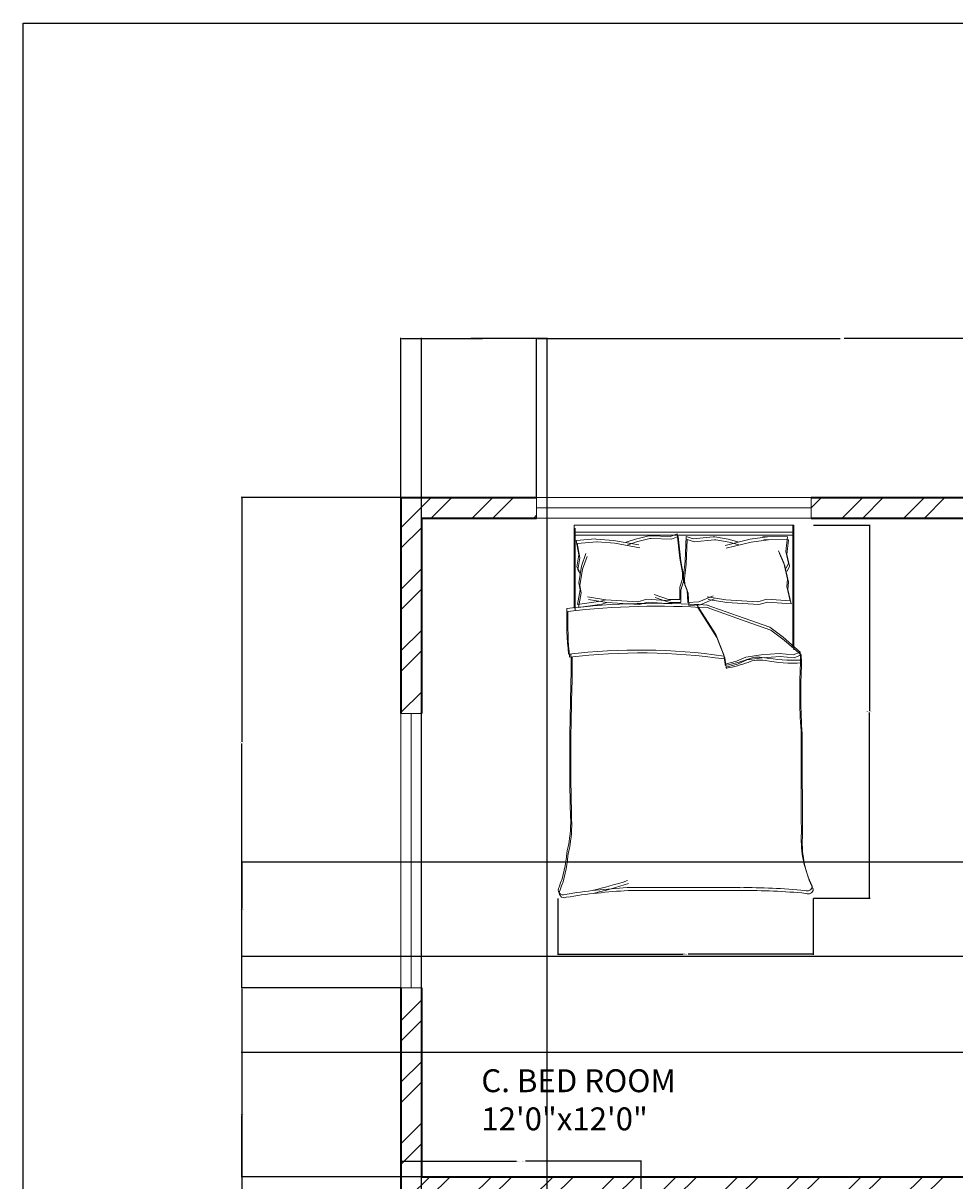
# Model space of a CAD drawing. Units: inches. Extents: x 1965 to 2673, y 1802 to 2669.
# Tile 9 of 16: x 1965 to 2168, y 2416 to 2669. Entities that reach past the tile are written whole.
import ezdxf

# ---------------------------------------------------------------- set-up
doc = ezdxf.new("R2010")
doc.units = ezdxf.units.IN
for name, color, linetype, lineweight in [('A-ANNO-DIMS', 2, 'Continuous', 18), ('A-ANNO-TTLB', 7, 'Continuous', 25), ('A-AREA-IDEN', 7, 'Continuous', 18), ('A-FURN', 8, 'Continuous', 13), ('A-GLAZ', 181, 'Continuous', 18), ('A-WALL', 7, 'Continuous', 35), ('A-WALL-PATT', 252, 'Continuous', 13)]:
    doc.layers.add(name, color=color, linetype=linetype, lineweight=lineweight)
doc.styles.get("Standard").update_dxf_attribs({"font": 'arial.ttf'})
doc.dimstyles.get("Standard").update_dxf_attribs({"dimtxt": 0.18, "dimasz": 0.18, "dimexe": 0.18, "dimexo": 0.0625, "dimgap": 0.09, "dimtad": 0, "dimtih": 1, "dimtoh": 1, "dimdec": 4, "dimzin": 0, "dimdsep": 46, "dimtxsty": 'Standard', "dimcen": 0.09, "dimadec": 0, "dimazin": 0, "dimtfac": 1, "dimtdec": 4, "dimtofl": 0, "dimtmove": 0, "dimatfit": 3, "dimfxl": 1, "dimtolj": 1, "dimtzin": 0, "dimarcsym": 0})

# ---------------------------------------------------------------- blocks, each defined once
blk = doc.blocks.new('BED-DOUBLE')
for p, q in [((3.47, 63.33), (3.47, 81.44)), ((3.47, 63.33), (3.47, 81.44)), ((3.47, 81.44), (51.49, 81.44)), ((51.26, 81.44), (51.26, 54.83)), ((51.26, 81.44), (51.26, 54.83)), ((51.49, 81.44), (51.49, 80.8)), ((3.47, 79.91), (51.26, 79.91)), ((3.47, 79.91), (51.26, 79.91)), ((3.7, 62.69), (3.7, 80.8)), ((3.7, 62.69), (3.7, 80.8)), ((3.7, 79.27), (51.49, 79.27)), ((3.7, 79.27), (51.49, 79.27)), ((16.87, 78.41), (19.76, 79.14)), ((16.87, 78.41), (19.76, 79.14)), ((17.1, 77.77), (19.99, 78.5)), ((17.1, 77.77), (19.99, 78.5)), ((19.76, 79.14), (20.09, 79.14)), ((19.76, 79.14), (20.09, 79.14)), ((19.99, 78.5), (20.31, 78.5)), ((19.99, 78.5), (20.31, 78.5)), ((20.09, 79.14), (24.53, 78.99)), ((20.09, 79.14), (24.53, 78.99)), ((20.31, 78.5), (24.76, 78.35)), ((20.31, 78.5), (24.76, 78.35)), ((24.53, 78.99), (25.98, 79.57)), ((24.53, 78.99), (25.98, 79.57)), ((24.76, 78.35), (26.21, 78.93)), ((24.76, 78.35), (26.21, 78.93)), ((25.98, 79.57), (26.56, 74.22)), ((25.98, 79.57), (26.56, 74.22)), ((26.21, 78.93), (26.78, 73.58)), ((26.21, 78.93), (26.78, 73.58)), ((27.97, 78.95), (27.73, 73.57)), ((27.97, 78.95), (27.73, 73.57)), ((29.45, 78.46), (27.97, 78.95)), ((29.45, 78.46), (27.97, 78.95)), ((33.88, 78.88), (29.45, 78.46)), ((33.88, 78.88), (29.45, 78.46)), ((34.2, 78.9), (33.88, 78.88)), ((34.2, 78.9), (33.88, 78.88)), ((37.13, 78.36), (34.2, 78.9)), ((37.13, 78.36), (34.2, 78.9)), ((45.71, 78.9), (41.91, 78.37)), ((45.71, 78.9), (41.91, 78.37)), ((50.11, 78.88), (44.7, 78.98)), ((44.7, 78.98), (45.71, 78.9)), ((50.11, 78.88), (44.7, 78.98)), ((44.7, 78.98), (45.71, 78.9)), ((50.11, 78.88), (49.73, 75.67)), ((50.11, 78.88), (49.73, 75.67)), ((51.49, 80.8), (51.49, 54.19)), ((51.49, 80.8), (51.49, 54.19)), ((3.89, 78.1), (8.17, 78.43)), ((3.89, 78.1), (8.17, 78.43)), ((3.89, 78.12), (4.47, 74.94)), ((3.89, 78.12), (4.47, 74.94)), ((4.12, 77.46), (8.4, 77.79)), ((4.12, 77.46), (8.4, 77.79)), ((4.12, 77.49), (4.7, 74.3)), ((4.12, 77.49), (4.7, 74.3)), ((8.17, 78.43), (8.28, 78.41)), ((8.17, 78.43), (8.28, 78.41)), ((8.28, 78.41), (12.1, 78.12)), ((8.28, 78.41), (12.1, 78.12)), ((8.4, 77.79), (8.51, 77.77)), ((8.4, 77.79), (8.51, 77.77)), ((8.51, 77.77), (12.33, 77.49)), ((8.51, 77.77), (12.33, 77.49)), ((12.1, 78.12), (17.6, 77.11)), ((12.1, 78.12), (17.6, 77.11)), ((12.33, 77.49), (17.82, 76.47)), ((12.33, 77.49), (17.82, 76.47)), ((14.85, 77.69), (16.87, 78.41)), ((14.85, 77.69), (16.87, 78.41)), ((15.08, 77.05), (17.1, 77.77)), ((15.08, 77.05), (17.1, 77.77)), ((28.2, 78.31), (27.96, 72.93)), ((28.2, 78.31), (27.96, 72.93)), ((29.68, 77.82), (28.2, 78.31)), ((29.68, 77.82), (28.2, 78.31)), ((34.11, 78.24), (29.68, 77.82)), ((34.11, 78.24), (29.68, 77.82)), ((34.43, 78.26), (34.11, 78.24)), ((34.43, 78.26), (34.11, 78.24)), ((37.36, 77.72), (34.43, 78.26)), ((37.36, 77.72), (34.43, 78.26)), ((41.91, 78.37), (36.49, 77.02)), ((41.91, 78.37), (36.49, 77.02)), ((42.14, 77.73), (36.72, 76.38)), ((42.14, 77.73), (36.72, 76.38)), ((39.2, 77.77), (37.13, 78.36)), ((39.19, 77.77), (37.13, 78.36)), ((39.42, 77.13), (37.36, 77.72)), ((39.42, 77.13), (37.36, 77.72)), ((45.94, 78.26), (42.14, 77.73)), ((45.94, 78.26), (42.14, 77.73)), ((50.34, 78.24), (44.93, 78.34)), ((44.93, 78.34), (45.94, 78.26)), ((50.34, 78.24), (44.93, 78.34)), ((44.93, 78.34), (45.94, 78.26)), ((50.34, 78.24), (49.96, 75.03)), ((50.34, 78.24), (49.96, 75.03)), ((4.47, 74.94), (4.03, 72.34)), ((4.47, 74.94), (4.03, 72.34)), ((4.7, 74.3), (4.26, 71.7)), ((4.7, 74.3), (4.26, 71.7)), ((5.05, 72.49), (6.06, 75.23)), ((5.05, 72.49), (6.06, 75.23)), ((5.27, 71.85), (6.29, 74.59)), ((5.27, 71.85), (6.29, 74.59)), ((26.56, 74.22), (27.13, 71.04)), ((26.56, 74.22), (27.13, 71.04)), ((26.78, 73.58), (27.36, 70.4)), ((26.78, 73.58), (27.36, 70.4)), ((27.73, 73.57), (27.35, 70.36)), ((27.73, 73.57), (27.35, 70.36)), ((49.3, 73.18), (48.12, 75.86)), ((49.3, 73.18), (48.12, 75.86)), ((49.53, 72.54), (48.35, 75.22)), ((49.53, 72.54), (48.35, 75.22)), ((49.73, 75.67), (50.32, 73.1)), ((49.73, 75.67), (50.32, 73.1)), ((49.96, 75.03), (50.55, 72.46)), ((49.96, 75.03), (50.55, 72.46)), ((4.03, 72.34), (4.61, 71.33)), ((4.03, 72.34), (4.61, 71.33)), ((4.26, 71.7), (4.84, 70.69)), ((4.26, 71.7), (4.84, 70.69)), ((4.47, 68.87), (5.05, 72.49)), ((4.47, 68.87), (5.05, 72.49)), ((4.7, 68.23), (5.27, 71.85)), ((4.7, 68.23), (5.27, 71.85)), ((27.13, 71.04), (27.13, 69.74)), ((27.13, 71.04), (27.13, 69.74)), ((27.96, 72.93), (27.58, 69.72)), ((27.96, 72.93), (27.58, 69.72)), ((50.11, 69.61), (49.3, 73.18)), ((50.11, 69.61), (49.3, 73.18)), ((50.34, 68.97), (49.53, 72.54)), ((50.34, 68.97), (49.53, 72.54)), ((50.32, 73.1), (49.81, 72.06)), ((50.32, 73.1), (49.81, 72.06)), ((50.55, 72.46), (50.04, 71.42)), ((50.55, 72.46), (50.04, 71.42)), ((4.76, 67.28), (4.47, 68.87)), ((4.76, 67.28), (4.47, 68.87)), ((27.13, 69.74), (26.56, 67.86)), ((27.13, 69.74), (26.56, 67.86)), ((27.36, 69.1), (26.78, 67.22)), ((27.36, 69.1), (26.78, 67.22)), ((27.35, 70.36), (27.43, 69.06)), ((27.35, 70.36), (27.43, 69.06)), ((27.36, 70.4), (27.36, 69.1)), ((27.36, 70.4), (27.36, 69.1)), ((27.43, 69.06), (28.13, 67.22)), ((27.43, 69.06), (28.13, 67.22)), ((27.58, 69.72), (27.66, 68.42)), ((27.58, 69.72), (27.66, 68.42)), ((27.66, 68.42), (28.35, 66.58)), ((27.66, 68.42), (28.35, 66.58)), ((49.92, 68.01), (50.11, 69.61)), ((49.92, 68.01), (50.11, 69.61)), ((50.15, 67.37), (50.34, 68.97)), ((50.15, 67.37), (50.34, 68.97)), ((4.18, 64.1), (4.76, 67.28)), ((4.18, 64.1), (4.76, 67.28)), ((4.41, 63.46), (4.99, 66.64)), ((4.41, 63.46), (4.99, 66.64)), ((4.99, 66.64), (4.7, 68.23)), ((4.99, 66.64), (4.7, 68.23)), ((6.38, 65.81), (10.41, 65.15)), ((6.38, 65.81), (10.41, 65.15)), ((24.1, 65.18), (20.95, 66.27)), ((24.1, 65.18), (20.95, 66.27)), ((26.56, 67.86), (26.56, 65.18)), ((26.56, 67.86), (26.56, 65.18)), ((26.78, 67.22), (26.78, 64.54)), ((26.78, 67.22), (26.78, 64.54)), ((28.13, 67.22), (28.29, 64.55)), ((28.13, 67.22), (28.29, 64.55)), ((28.35, 66.58), (28.52, 63.91)), ((28.35, 66.58), (28.52, 63.91)), ((30.75, 64.7), (33.82, 65.99)), ((30.75, 64.7), (33.82, 65.99)), ((32.56, 65.81), (36.59, 65.15)), ((32.56, 65.81), (36.59, 65.15)), ((50.69, 64.87), (49.92, 68.01)), ((50.69, 64.87), (49.92, 68.01)), ((50.92, 64.23), (50.15, 67.37)), ((50.92, 64.23), (50.15, 67.37)), ((9.28, 64.82), (4.18, 64.1)), ((9.28, 64.82), (4.18, 64.1)), ((9.5, 64.18), (4.41, 63.46)), ((9.5, 64.18), (4.41, 63.46)), ((6.6, 65.17), (10.64, 64.51)), ((6.61, 65.17), (10.64, 64.51)), ((10.41, 65.15), (9.28, 64.82)), ((10.41, 65.15), (9.28, 64.82)), ((10.64, 64.51), (9.5, 64.18)), ((10.64, 64.51), (9.5, 64.18)), ((10.41, 65.15), (17.42, 64.71)), ((10.41, 65.15), (17.42, 64.71)), ((10.64, 64.51), (17.65, 64.08)), ((10.64, 64.51), (17.65, 64.08)), ((17.42, 64.71), (19.38, 65.27)), ((17.42, 64.71), (19.38, 65.27)), ((17.65, 64.08), (19.61, 64.63)), ((17.65, 64.08), (19.61, 64.63)), ((19.38, 65.27), (24.51, 64.87)), ((19.38, 65.27), (24.51, 64.87)), ((19.61, 64.63), (24.74, 64.23)), ((19.61, 64.63), (24.74, 64.23)), ((24.33, 64.54), (21.18, 65.63)), ((24.33, 64.54), (21.18, 65.63)), ((26.56, 65.18), (24.1, 65.18)), ((26.56, 65.18), (24.1, 65.18)), ((26.78, 64.54), (24.33, 64.54)), ((26.78, 64.54), (24.33, 64.54)), ((28.29, 64.55), (30.75, 64.7)), ((28.29, 64.55), (30.75, 64.7)), ((28.52, 63.91), (30.97, 64.06)), ((28.52, 63.91), (30.97, 64.06)), ((30.25, 64.06), (34.44, 57.56)), ((30.25, 64.06), (34.44, 57.56)), ((30.48, 63.42), (34.67, 56.92)), ((30.48, 63.42), (34.67, 56.92)), ((30.97, 64.06), (34.04, 65.35)), ((30.97, 64.06), (34.04, 65.35)), ((40.64, 61.12), (32.3, 64.06)), ((40.64, 61.12), (32.3, 64.06)), ((40.87, 60.48), (32.53, 63.42)), ((40.87, 60.48), (32.53, 63.42)), ((32.79, 65.17), (36.82, 64.51)), ((32.79, 65.17), (36.82, 64.51)), ((36.59, 65.15), (43.6, 64.71)), ((36.59, 65.15), (43.6, 64.71)), ((36.82, 64.51), (43.83, 64.08)), ((36.82, 64.51), (43.83, 64.08)), ((43.6, 64.71), (45.56, 65.27)), ((43.6, 64.71), (45.56, 65.27)), ((43.83, 64.08), (45.79, 64.63)), ((43.83, 64.08), (45.79, 64.63)), ((45.56, 65.27), (50.69, 64.87)), ((45.56, 65.27), (50.69, 64.87)), ((45.79, 64.63), (50.92, 64.23)), ((45.79, 64.63), (50.92, 64.23)), ((46.21, 59.11), (40.64, 61.12)), ((46.21, 59.11), (40.64, 61.12)), ((46.44, 58.47), (40.87, 60.48)), ((46.44, 58.47), (40.87, 60.48)), ((49.16, 56.95), (46.21, 59.11)), ((49.16, 56.95), (46.21, 59.11)), ((49.39, 56.31), (46.44, 58.47)), ((49.39, 56.31), (46.44, 58.47)), ((34.44, 57.56), (36.15, 53.08)), ((34.44, 57.56), (36.15, 53.08)), ((34.67, 56.92), (36.38, 52.44)), ((34.67, 56.92), (36.38, 52.44)), ((52.86, 53.69), (49.16, 56.95)), ((52.86, 53.69), (49.16, 56.95)), ((53.09, 53.06), (49.39, 56.31)), ((53.09, 53.06), (49.39, 56.31)), ((44.36, 53.08), (48.23, 53.39)), ((44.36, 53.08), (48.23, 53.39)), ((48.23, 53.39), (51.33, 53.08)), ((48.23, 53.39), (51.33, 53.08)), ((51.33, 53.08), (52.86, 53.69)), ((51.33, 53.08), (52.86, 53.69)), ((52.94, 51.95), (52.86, 53.69, 3.87)), ((52.94, 51.95), (52.86, 53.69, 3.87)), ((36.15, 53.08), (36.46, 51.06)), ((36.15, 53.08), (36.46, 51.06)), ((36.38, 52.44), (36.69, 50.42)), ((36.38, 52.44), (36.69, 50.42)), ((36.46, 51.06), (38.94, 51.68)), ((36.46, 51.06), (38.94, 51.68)), ((36.69, 50.42), (39.16, 51.04)), ((36.69, 50.42), (39.16, 51.04)), ((38.94, 51.68), (40.95, 52.61)), ((38.94, 51.68), (40.95, 52.61)), ((39.16, 51.04), (41.18, 51.97)), ((39.16, 51.04), (41.18, 51.97)), ((40.95, 52.61), (44.36, 53.08)), ((40.95, 52.61), (44.36, 53.08)), ((41.18, 51.97), (44.58, 52.44)), ((41.18, 51.97), (44.58, 52.44)), ((44.58, 52.44), (48.46, 52.75)), ((44.58, 52.44), (48.46, 52.75)), ((48.46, 52.75), (51.55, 52.44)), ((48.46, 52.75), (51.55, 52.44)), ((51.55, 52.44), (53.09, 53.06)), ((51.55, 52.44), (53.09, 53.06)), ((53.17, 51.31), (53.09, 53.06, 3.87)), ((53.17, 51.31), (53.09, 53.06, 3.87)), ((15.06, 2.2), (39.67, 2.2)), ((15.06, 2.2), (39.67, 2.2)), ((15.29, 1.56), (39.9, 1.56)), ((15.29, 1.56), (39.9, 1.56))]:
    blk.add_line(p, q)
for centre, radius, start, end in [((21.35, -100.61), 164.97, 86.0865, 96.7821), ((21.35, -100.61), 164.97, 86.0865, 96.7821), ((21.58, -101.25), 164.97, 86.0865, 96.7821), ((21.58, -101.25), 164.97, 86.0865, 96.7821), ((85.16, 61.34), 83.31, 178.7218, 185.604), ((85.16, 61.34), 83.31, 178.7218, 185.604), ((85.39, 60.71), 83.31, 178.7218, 185.604), ((85.38, 60.71), 83.31, 178.7218, 185.604), ((17.75, -74.88), 129.02, 81.7845, 96.9006), ((17.75, -74.88), 129.02, 81.7845, 96.9006), ((17.98, -75.51), 129.02, 81.7845, 96.9006), ((17.98, -75.51), 129.02, 81.7845, 96.9006), ((-167.31, 50.27), 170.11, 358.4762, 1.0082), ((-167.31, 50.27), 170.11, 358.4762, 1.0082), ((-167.08, 49.63), 170.11, 358.4762, 1.0082), ((-167.08, 49.63), 170.11, 358.4762, 1.0082), ((36.63, 51), 0.185, 160.2464, 271.1377), ((36.63, 51), 0.185, 160.2464, 271.1377), ((31.15, 79.96), 29.65, 280.6617, 289.8806), ((31.15, 79.96), 29.65, 280.6617, 289.8806), ((31.38, 79.32), 29.65, 280.6617, 289.8806), ((31.38, 79.32), 29.65, 280.6617, 289.8806), ((43.74, 46.37), 6.22, 78.6608, 113.7384), ((43.74, 46.37), 6.22, 78.6608, 113.7384), ((43.97, 45.74), 6.22, 78.6608, 113.7384), ((43.97, 45.74), 6.22, 78.6608, 113.7384), ((51.32, 88.1), 36.18, 259.8763, 272.5657), ((51.32, 88.1), 36.18, 259.8763, 272.5657), ((51.55, 87.46), 36.18, 259.8763, 272.5657), ((51.55, 87.46), 36.18, 259.8763, 272.5657), ((182.26, 45.13), 129.5, 176.9791, 183.8365), ((182.26, 45.13), 129.5, 176.9791, 183.8365), ((182.49, 44.49), 129.5, 176.9791, 183.8365), ((182.49, 44.49), 129.5, 176.9791, 183.8365), ((36.86, 50.36), 0.185, 160.2464, 271.1377), ((36.86, 50.36), 0.185, 160.2464, 271.1377), ((484.82, 30.83), 482.31, 178.2277, 181.7185), ((484.82, 30.83), 482.31, 178.2277, 181.7185), ((485.05, 30.19), 482.31, 178.2277, 181.7185), ((485.05, 30.19), 482.31, 178.2277, 181.7185), ((-4508.75, 13.62), 4561.86, 0.00217, 0.28689), ((-4508.75, 13.62), 4561.86, 0.00217, 0.28689), ((-4508.52, 12.98), 4561.86, 0.00217, 0.28689), ((-4508.52, 12.98), 4561.86, 0.00217, 0.28689), ((-26.9, 16.93), 29.63, 346.0648, 358.9113), ((-26.9, 16.93), 29.63, 346.0648, 358.9113), ((-26.68, 16.29), 29.63, 346.0648, 358.9113), ((-26.68, 16.29), 29.63, 346.0648, 358.9113), ((76.15, 12.77), 23.07, 177.4714, 206.4681), ((76.15, 12.77), 23.07, 177.4714, 206.4681), ((76.38, 12.14), 23.07, 177.4714, 206.4681), ((76.38, 12.14), 23.07, 177.4714, 206.4681), ((-21.66, 11.17), 23.56, 337.9751, 356.652), ((-21.66, 11.17), 23.56, 337.9751, 356.652), ((-21.44, 10.53), 23.56, 337.9751, 356.652), ((-21.44, 10.53), 23.56, 337.9751, 356.652), ((-17.23, 105.15), 106.46, 283.3832, 287.7053), ((-17.23, 105.15), 106.46, 283.3832, 287.7053), ((-17, 104.51), 106.46, 283.3832, 287.7053), ((-17, 104.51), 106.46, 283.3832, 287.7053), ((1.08, 1.72), 1.09, 146.1736, 293.4781), ((1.08, 1.72), 1.09, 146.1736, 293.4781), ((1.31, 1.08), 1.09, 146.1736, 293.4781), ((1.31, 1.08), 1.09, 146.1736, 293.4781), ((21.42, -119.4), 121.76, 92.9958, 99.4091), ((21.42, -119.4), 121.76, 92.9958, 99.4091), ((21.65, -120.04), 121.76, 92.9958, 99.4091), ((21.65, -120.04), 121.76, 92.9958, 99.4091), ((41.15, -130.84), 133.04, 84.4998, 90.6351), ((41.15, -130.84), 133.04, 84.4998, 90.6351), ((41.38, -131.48), 133.04, 84.4998, 90.6351), ((41.37, -131.48), 133.04, 84.4998, 90.6351), ((54.4, 2.57), 1.1, 242.6588, 356.02), ((54.4, 2.57), 1.1, 242.6588, 356.02), ((54.63, 1.93), 1.1, 242.6588, 356.02), ((54.63, 1.93), 1.1, 242.6588, 356.02)]:
    blk.add_arc(centre, radius, start, end)
blk = doc.blocks.new('WIN-60IN')
for p, q in [((0, 4.5), (0, 0)), ((0, 4.5), (60, 4.5)), ((60, 2.25), (60, 4.5)), ((60, 4.5), (60, 0)), ((0, 0), (0, 2.25)), ((0, 2.25), (60, 2.25)), ((60, 0), (0, 0))]:
    blk.add_line(p, q)
blk = doc.blocks.new('*D15')
at = {"layer": 'A-ANNO-DIMS', "color": 0, "lineweight": -2, "transparency": 16777216}
for p, q in [((2137.28, 2559.53), (2149.63, 2559.53)), ((2149.45, 2559.35), (2149.45, 2518.94)), ((2149.45, 2478.16), (2149.45, 2518.57)), ((2137.28, 2477.98), (2149.63, 2477.98))]:
    blk.add_line(p, q, dxfattribs=at)
at = {"layer": 'A-ANNO-DIMS', "color": 0, "transparency": 16777216}
for points in [[(2149.42, 2559.35), (2149.48, 2559.35), (2149.45, 2559.53)], [(2149.42, 2478.16), (2149.48, 2478.16), (2149.45, 2477.98)]]:
    blk.add_solid(points, dxfattribs=at)
at = {"layer": 'Defpoints', "color": 0, "transparency": 16777216}
for p in [(2137.21, 2559.53), (2149.45, 2559.53), (2137.21, 2477.98)]:
    blk.add_point(p, dxfattribs=at)
at = {"layer": 'A-ANNO-DIMS', "color": 0, "transparency": 16777216, "insert": (2149.45, 2518.76), "char_height": 0.18, "attachment_point": 5}
blk.add_mtext('\\A1;BED 82 TYP.', dxfattribs=at)
blk = doc.blocks.new('*D16')
at = {"layer": 'A-ANNO-DIMS', "color": 0, "lineweight": -2, "transparency": 16777216}
for p, q in [((2081.39, 2477.92), (2081.39, 2465.57)), ((2137.21, 2477.92), (2137.21, 2465.57)), ((2081.57, 2465.75), (2108.77, 2465.75)), ((2137.03, 2465.75), (2109.83, 2465.75))]:
    blk.add_line(p, q, dxfattribs=at)
at = {"layer": 'A-ANNO-DIMS', "color": 0, "transparency": 16777216}
for points in [[(2081.57, 2465.78), (2081.57, 2465.72), (2081.39, 2465.75)], [(2137.03, 2465.78), (2137.03, 2465.72), (2137.21, 2465.75)]]:
    blk.add_solid(points, dxfattribs=at)
at = {"layer": 'Defpoints', "color": 0, "transparency": 16777216}
for p in [(2081.39, 2477.98), (2137.21, 2477.98), (2137.21, 2465.75)]:
    blk.add_point(p, dxfattribs=at)
at = {"layer": 'A-ANNO-DIMS', "color": 0, "transparency": 16777216, "insert": (2109.3, 2465.75), "char_height": 0.18, "attachment_point": 5}
blk.add_mtext('\\A1;56 TYP.', dxfattribs=at)
blk = doc.blocks.new('*D23')
at = {"layer": 'A-ANNO-DIMS', "color": 0, "lineweight": -2, "transparency": 16777216}
for p, q in [((2047.09, 2412.65), (2047.09, 2420.65)), ((2047.27, 2420.47), (2072.37, 2420.47)), ((2099.41, 2420.47), (2074.32, 2420.47)), ((2099.59, 2412.65), (2099.59, 2420.65))]:
    blk.add_line(p, q, dxfattribs=at)
at = {"layer": 'A-ANNO-DIMS', "color": 0, "transparency": 16777216}
for points in [[(2047.27, 2420.5), (2047.27, 2420.44), (2047.09, 2420.47)], [(2099.41, 2420.5), (2099.41, 2420.44), (2099.59, 2420.47)]]:
    blk.add_solid(points, dxfattribs=at)
at = {"layer": 'Defpoints', "color": 0, "transparency": 16777216}
for p in [(2099.59, 2420.47), (2047.09, 2412.59), (2099.59, 2412.59)]:
    blk.add_point(p, dxfattribs=at)
at = {"layer": 'A-ANNO-DIMS', "color": 0, "transparency": 16777216, "insert": (2073.34, 2420.47), "char_height": 0.18, "attachment_point": 5}
blk.add_mtext('\\A1;SHAFT 53 TYP.', dxfattribs=at)
blk = doc.blocks.new('*D27')
at = {"layer": 'A-ANNO-DIMS', "color": 0, "lineweight": -2, "transparency": 16777216}
for p, q in [((2047.09, 2565.65), (2047.09, 2600.5)), ((2047.27, 2600.32), (2061.46, 2600.32)), ((2076.58, 2600.32), (2062.39, 2600.32)), ((2076.76, 2565.65), (2076.76, 2600.5))]:
    blk.add_line(p, q, dxfattribs=at)
at = {"layer": 'A-ANNO-DIMS', "color": 0, "transparency": 16777216}
for points in [[(2047.27, 2600.35), (2047.27, 2600.29), (2047.09, 2600.32)], [(2076.58, 2600.35), (2076.58, 2600.29), (2076.76, 2600.32)]]:
    blk.add_solid(points, dxfattribs=at)
at = {"layer": 'Defpoints', "color": 0, "transparency": 16777216}
for p in [(2076.76, 2600.32), (2047.09, 2565.59), (2076.76, 2565.59)]:
    blk.add_point(p, dxfattribs=at)
at = {"layer": 'A-ANNO-DIMS', "color": 0, "transparency": 16777216, "insert": (2061.92, 2600.32), "char_height": 0.18, "attachment_point": 5}
blk.add_mtext('\\A1;29.663', dxfattribs=at)
blk = doc.blocks.new('*D28')
at = {"layer": 'A-ANNO-DIMS', "color": 0, "lineweight": -2, "transparency": 16777216}
for p, q in [((2076.76, 2565.65), (2076.76, 2600.5)), ((2076.94, 2600.32), (2143.04, 2600.32)), ((2210.05, 2600.32), (2143.95, 2600.32)), ((2210.23, 2565.65), (2210.23, 2600.5))]:
    blk.add_line(p, q, dxfattribs=at)
at = {"layer": 'A-ANNO-DIMS', "color": 0, "transparency": 16777216}
for points in [[(2076.94, 2600.35), (2076.94, 2600.29), (2076.76, 2600.32)], [(2210.05, 2600.35), (2210.05, 2600.29), (2210.23, 2600.32)]]:
    blk.add_solid(points, dxfattribs=at)
at = {"layer": 'Defpoints', "color": 0, "transparency": 16777216}
for p in [(2210.23, 2600.32), (2076.76, 2565.59), (2210.23, 2565.59)]:
    blk.add_point(p, dxfattribs=at)
at = {"layer": 'A-ANNO-DIMS', "color": 0, "transparency": 16777216, "insert": (2143.49, 2600.32), "char_height": 0.18, "attachment_point": 5}
blk.add_mtext('\\A1;133.48', dxfattribs=at)
blk = doc.blocks.new('*D37')
at = {"layer": 'A-ANNO-DIMS', "color": 0, "lineweight": -2, "transparency": 16777216}
for p, q in [((2047.03, 2458.38), (2012.19, 2458.38)), ((2012.37, 2458.2), (2012.37, 2383.91)), ((2012.37, 2309.25), (2012.37, 2383.54)), ((2047.03, 2309.07), (2012.19, 2309.07))]:
    blk.add_line(p, q, dxfattribs=at)
at = {"layer": 'A-ANNO-DIMS', "color": 0, "transparency": 16777216}
for points in [[(2012.34, 2458.2), (2012.4, 2458.2), (2012.37, 2458.38)], [(2012.34, 2309.25), (2012.4, 2309.25), (2012.37, 2309.07)]]:
    blk.add_solid(points, dxfattribs=at)
at = {"layer": 'Defpoints', "color": 0, "transparency": 16777216}
for p in [(2012.37, 2458.38), (2047.09, 2458.38), (2047.09, 2309.07)]:
    blk.add_point(p, dxfattribs=at)
at = {"layer": 'A-ANNO-DIMS', "color": 0, "transparency": 16777216, "insert": (2012.37, 2383.73), "char_height": 0.18, "attachment_point": 5}
blk.add_mtext('\\A1;149.3', dxfattribs=at)
blk = doc.blocks.new('*D38')
at = {"layer": 'A-ANNO-DIMS', "color": 0, "lineweight": -2, "transparency": 16777216}
for p, q in [((2047.03, 2565.59), (2012.19, 2565.59)), ((2012.37, 2565.41), (2012.37, 2512.17)), ((2012.37, 2458.56), (2012.37, 2511.8)), ((2047.03, 2458.38), (2012.19, 2458.38))]:
    blk.add_line(p, q, dxfattribs=at)
at = {"layer": 'A-ANNO-DIMS', "color": 0, "transparency": 16777216}
for points in [[(2012.34, 2565.41), (2012.4, 2565.41), (2012.37, 2565.59)], [(2012.34, 2458.56), (2012.4, 2458.56), (2012.37, 2458.38)]]:
    blk.add_solid(points, dxfattribs=at)
at = {"layer": 'Defpoints', "color": 0, "transparency": 16777216}
for p in [(2012.37, 2565.59), (2047.09, 2565.59), (2047.09, 2458.38)]:
    blk.add_point(p, dxfattribs=at)
at = {"layer": 'A-ANNO-DIMS', "color": 0, "transparency": 16777216, "insert": (2012.37, 2511.99), "char_height": 0.18, "attachment_point": 5}
blk.add_mtext('\\A1;107.2', dxfattribs=at)
blk = doc.blocks.new('*D39')
at = {"layer": 'A-ANNO-DIMS', "color": 0, "lineweight": -2, "transparency": 16777216}
for p, q in [((2051.59, 1936.15), (2051.59, 2600.5)), ((2051.77, 2600.32), (2064.93, 2600.32)), ((2078.87, 2600.32), (2065.72, 2600.32)), ((2079.05, 1936.15), (2079.05, 2600.5))]:
    blk.add_line(p, q, dxfattribs=at)
at = {"layer": 'A-ANNO-DIMS', "color": 0, "transparency": 16777216}
for points in [[(2051.77, 2600.35), (2051.77, 2600.29), (2051.59, 2600.32)], [(2078.87, 2600.35), (2078.87, 2600.29), (2079.05, 2600.32)]]:
    blk.add_solid(points, dxfattribs=at)
at = {"layer": 'Defpoints', "color": 0, "transparency": 16777216}
for p in [(2079.05, 2600.32), (2051.59, 1936.09), (2079.05, 1936.09)]:
    blk.add_point(p, dxfattribs=at)
at = {"layer": 'A-ANNO-DIMS', "color": 0, "transparency": 16777216, "insert": (2065.32, 2600.32), "char_height": 0.18, "attachment_point": 5}
blk.add_mtext('\\A1;27.46', dxfattribs=at)
blk = doc.blocks.new('*D49')
at = {"layer": 'A-ANNO-DIMS', "color": 0, "lineweight": -2, "transparency": 16777216}
for p, q in [((2573.53, 2444.23), (2012.19, 2444.23)), ((2012.37, 2444.05), (2012.37, 2430.84)), ((2012.37, 2417.27), (2012.37, 2430.48)), ((2573.53, 2417.09), (2012.19, 2417.09))]:
    blk.add_line(p, q, dxfattribs=at)
at = {"layer": 'A-ANNO-DIMS', "color": 0, "transparency": 16777216}
for points in [[(2012.34, 2444.05), (2012.4, 2444.05), (2012.37, 2444.23)], [(2012.34, 2417.27), (2012.4, 2417.27), (2012.37, 2417.09)]]:
    blk.add_solid(points, dxfattribs=at)
at = {"layer": 'Defpoints', "color": 0, "transparency": 16777216}
for p in [(2012.37, 2444.23), (2573.59, 2444.23), (2573.59, 2417.09)]:
    blk.add_point(p, dxfattribs=at)
at = {"layer": 'A-ANNO-DIMS', "color": 0, "transparency": 16777216, "insert": (2012.37, 2430.66), "char_height": 0.18, "attachment_point": 5}
blk.add_mtext('\\A1;27.137', dxfattribs=at)
blk = doc.blocks.new('*D54')
at = {"layer": 'A-ANNO-DIMS', "color": 0, "lineweight": -2, "transparency": 16777216}
for p, q in [((2195.53, 2485.86), (2012.19, 2485.86)), ((2012.37, 2485.68), (2012.37, 2475.73)), ((2012.37, 2465.42), (2012.37, 2475.37)), ((2195.53, 2465.24), (2012.19, 2465.24))]:
    blk.add_line(p, q, dxfattribs=at)
at = {"layer": 'A-ANNO-DIMS', "color": 0, "transparency": 16777216}
for points in [[(2012.34, 2485.68), (2012.4, 2485.68), (2012.37, 2485.86)], [(2012.34, 2465.42), (2012.4, 2465.42), (2012.37, 2465.24)]]:
    blk.add_solid(points, dxfattribs=at)
at = {"layer": 'Defpoints', "color": 0, "transparency": 16777216}
for p in [(2012.37, 2485.86), (2195.59, 2485.86), (2195.59, 2465.24)]:
    blk.add_point(p, dxfattribs=at)
at = {"layer": 'A-ANNO-DIMS', "color": 0, "transparency": 16777216, "insert": (2012.37, 2475.55), "char_height": 0.18, "attachment_point": 5}
blk.add_mtext('\\A1;20.625', dxfattribs=at)

msp = doc.modelspace()

# ---------------------------------------------------------------- hatches: boundary and pattern name
at = {"layer": 'A-WALL-PATT'}
h = msp.add_hatch(dxfattribs=at)
h.set_pattern_fill('ANSI32', color=256)
h.paths.add_polyline_path([(2051.5927, 2561.0914), (2076.7559, 2561.0914), (2076.7559, 2563.3414), (2076.7559, 2565.5914), (2047.0927, 2565.5914), (2047.0927, 2518.3824), (2051.5927, 2518.3824)])
h.paths.add_polyline_path([(2051.5927, 2458.3824), (2049.3427, 2458.3824), (2047.0927, 2458.3824), (2047.0927, 2412.5914), (2248.0927, 2412.5914), (2248.0927, 2268.5914), (2252.5927, 2268.5914), (2252.5927, 2412.5914), (2252.5927, 2421.0404), (2250.3427, 2421.0404), (2248.0927, 2421.0404), (2248.0927, 2417.0914), (2051.5927, 2417.0914)])
h.paths.add_polyline_path([(2211.4933, 2268.5914), (2104.0927, 2268.5914), (2104.0927, 2272.4654), (2101.8427, 2272.4654), (2099.5927, 2272.4654), (2099.5927, 2268.5914), (2051.5927, 2268.5914), (2051.5927, 2264.0914), (2147.5927, 2264.0914), (2147.5927, 2259.8893), (2152.0927, 2259.8893), (2152.0927, 2264.0914), (2211.4933, 2264.0914), (2211.4933, 2266.3414)])
h.paths.add_polyline_path([(2104.0927, 2376.0914), (2099.5927, 2376.0914), (2047.0927, 2376.0914), (2047.0927, 2333.0682), (2051.5927, 2333.0682), (2051.5927, 2371.5914), (2099.5927, 2371.5914), (2099.5927, 2293.6123), (2104.0927, 2293.6123)], flags=17)
h.paths.add_polyline_path([(2051.5927, 2309.0682), (2047.0927, 2309.0682), (2047.0927, 2233.5821), (2051.5927, 2233.5821)])
h.paths.add_polyline_path([(2104.0927, 2412.5914), (2099.5927, 2412.5914), (2099.5927, 2376.0914), (2104.0927, 2376.0914)], flags=17)
h.paths.add_polyline_path([(2290.1254, 2268.5914), (2242.4924, 2268.5914), (2242.4924, 2264.0914), (2290.1254, 2264.0914), (2290.1254, 2266.3414)])
h.paths.add_polyline_path([(2284.653, 2264.0914), (2280.153, 2264.0914), (2280.153, 2161.6826), (2284.653, 2161.6826)])
h.paths.add_polyline_path([(2578.0927, 2329.4656), (2573.5927, 2329.4656), (2573.5927, 2268.5914), (2525.5927, 2268.5914), (2525.5927, 2271.9222), (2523.3427, 2271.9222), (2521.0927, 2271.9222), (2521.0927, 2268.5914), (2324.2835, 2268.5914), (2324.2835, 2264.0914), (2329.0927, 2264.0914), (2329.0927, 2259.4977), (2333.5927, 2259.4977), (2333.5927, 2264.0914), (2473.0927, 2264.0914), (2473.0927, 2259.9371), (2477.5927, 2259.9371), (2477.5927, 2264.0914), (2573.5927, 2264.0914), (2573.5927, 2235.5751), (2578.0927, 2235.5751)])
h.paths.add_polyline_path([(2377.0927, 2412.5914), (2578.0927, 2412.5914), (2578.0927, 2444.2286), (2575.8427, 2444.2286), (2573.5927, 2444.2286), (2573.5927, 2417.0914), (2429.5927, 2417.0914), (2377.0927, 2417.0914), (2377.0927, 2421.7443), (2372.5927, 2421.7443), (2372.5927, 2268.5914), (2377.0927, 2268.5914)])
h.paths.add_polyline_path([(2525.5927, 2371.5914), (2573.5927, 2371.5914), (2573.5927, 2353.4656), (2578.0927, 2353.4656), (2578.0927, 2376.0914), (2525.5927, 2376.0914), (2521.0927, 2376.0914), (2521.0927, 2290.6472), (2525.5927, 2290.6472)], flags=17)
h.paths.add_polyline_path([(2477.5927, 2236.4106), (2475.3427, 2236.4106), (2473.0927, 2236.4106), (2473.0927, 2084.5914), (2465.3309, 2084.5914), (2465.3309, 2080.0914), (2481.6764, 2080.0914), (2481.6764, 2082.3414), (2481.6764, 2084.5914), (2477.5927, 2084.5914), (2477.5927, 2151.5914), (2573.5927, 2151.5914), (2573.5927, 2130.2907), (2578.0927, 2130.2907), (2578.0927, 2199.5751), (2575.8427, 2199.5751), (2573.5927, 2199.5751), (2573.5927, 2156.0914), (2477.5927, 2156.0914)])
h.paths.add_polyline_path([(2573.5927, 2084.5914), (2505.5513, 2084.5914), (2505.5513, 2080.0914), (2573.5927, 2080.0914)], flags=17)
h.paths.add_polyline_path([(2578.0927, 2106.2907), (2575.8427, 2106.2907), (2573.5927, 2106.2907), (2573.5927, 2050.8986), (2578.0927, 2050.8986)])
h.paths.add_polyline_path([(2578.0927, 1990.8986), (2575.8427, 1990.8986), (2573.5927, 1990.8986), (2573.5927, 1936.0914), (2522.132, 1936.0914), (2522.132, 1931.5914), (2578.0927, 1931.5914)])
h.paths.add_polyline_path([(2462.132, 1936.0914), (2429.5927, 1936.0914), (2429.5927, 2080.0914), (2432.623, 2080.0914), (2432.623, 2082.3414), (2432.623, 2084.5914), (2429.5927, 2084.5914), (2429.5927, 2120.5914), (2333.5927, 2120.5914), (2333.5927, 2229.3125), (2331.3427, 2229.3125), (2329.0927, 2229.3125), (2329.0927, 2116.0914), (2425.0927, 2116.0914), (2425.0927, 1936.0914), (2346.4058, 1936.0914), (2346.4058, 1931.5914), (2462.132, 1931.5914), (2462.132, 1933.8414)])
h.paths.add_polyline_path([(2211.767, 1933.8414), (2211.767, 1936.0914), (2200.0927, 1936.0914), (2200.0927, 2080.0914), (2200.0927, 2116.0914), (2284.653, 2116.0914), (2284.653, 2130.591), (2282.403, 2130.591), (2280.153, 2130.591), (2280.153, 2120.5914), (2200.0927, 2120.5914), (2195.5927, 2120.5914), (2195.5927, 2080.0914), (2195.5927, 1936.0914), (2139.0533, 1936.0914), (2139.0533, 1931.5914), (2211.767, 1931.5914)])
h.paths.add_polyline_path([(2282.2502, 1933.8414), (2282.2502, 1936.0914), (2259.767, 1936.0914), (2259.767, 1931.5914), (2282.2502, 1931.5914)], flags=17)
h.paths.add_polyline_path([(2051.5927, 1987.096), (2049.3427, 1987.096), (2047.0927, 1987.096), (2047.0927, 1931.5914), (2079.0533, 1931.5914), (2079.0533, 1933.8414), (2079.0533, 1936.0914), (2051.5927, 1936.0914)])
h.paths.add_polyline_path([(2051.5927, 2197.5821), (2049.3427, 2197.5821), (2047.0927, 2197.5821), (2047.0927, 2141.952), (2051.5927, 2141.952), (2051.5927, 2151.5914), (2147.5927, 2151.5914), (2147.5927, 2084.5914), (2144.3652, 2084.5914), (2144.3652, 2080.0914), (2155.9662, 2080.0914), (2155.9662, 2082.3414), (2155.9662, 2084.5914), (2152.0927, 2084.5914), (2152.0927, 2239.4921), (2149.8427, 2239.4921), (2147.5927, 2239.4921), (2147.5927, 2156.0914), (2051.5927, 2156.0914)])
h.paths.add_polyline_path([(2051.5927, 2080.0914), (2123.8575, 2080.0914), (2123.8575, 2082.3414), (2123.8575, 2084.5914), (2051.5927, 2084.5914), (2051.5927, 2117.952), (2047.0927, 2117.952), (2047.0927, 2047.096), (2051.5927, 2047.096)])
h = msp.add_hatch(dxfattribs=at)
h.set_pattern_fill('ANSI32', color=256)
h.paths.add_polyline_path([(2210.2316, 2563.3414), (2210.2316, 2565.5914), (2136.7559, 2565.5914), (2136.7559, 2561.0914), (2195.5927, 2561.0914), (2195.5927, 2485.8604), (2200.0927, 2485.8604), (2200.0927, 2561.0914), (2210.2316, 2561.0914)])
h.paths.add_polyline_path([(2285.9734, 2565.5914), (2234.2316, 2565.5914), (2234.2316, 2561.0914), (2248.0927, 2561.0914), (2248.0927, 2462.0914), (2200.0927, 2462.0914), (2200.0927, 2465.2357), (2197.8427, 2465.2357), (2195.5927, 2465.2357), (2195.5927, 2457.5914), (2248.0927, 2457.5914), (2248.0927, 2452.628), (2252.5927, 2452.628), (2252.5927, 2457.5914), (2257.5156, 2457.5914), (2257.5156, 2459.8414), (2257.5156, 2462.0914), (2252.5927, 2462.0914), (2252.5927, 2561.0914), (2285.9734, 2561.0914)])
h.paths.add_polyline_path([(2213.1374, 1872.8885), (2461.061, 1872.8885), (2461.061, 1909.9813), (2213.1374, 1909.9813)], flags=9)
h.paths.add_polyline_path([(2328.4056, 1942.3944), (2340.6089, 1942.3944), (2340.6089, 1952.6979), (2328.4056, 1952.6979)], flags=9)
h.paths.add_polyline_path([(2353.5759, 2030.9808), (2376.6455, 2030.9808), (2376.6455, 2041.2844), (2353.5759, 2041.2844)], flags=9)
h.paths.add_polyline_path([(2289.989, 2074.1041), (2326.916, 2074.1041), (2326.916, 2092.7615), (2289.989, 2092.7615)], flags=9)
h.paths.add_polyline_path([(2497.9, 2052.8638), (2548.3741, 2052.8638), (2548.3741, 2071.5212), (2497.9, 2071.5212)], flags=9)
h.paths.add_polyline_path([(2486.59, 2116.4883), (2515.7475, 2116.4883), (2515.7475, 2135.1456), (2486.59, 2135.1456)], flags=9)
h.paths.add_polyline_path([(2497.3007, 2181.2877), (2530.459, 2181.2877), (2530.459, 2199.945), (2497.3007, 2199.945)], flags=9)
h.paths.add_polyline_path([(2288.237, 2190.3228), (2324.1238, 2190.3228), (2324.1238, 2208.9802), (2288.237, 2208.9802)], flags=9)
h.paths.add_polyline_path([(2350.806, 2127.8307), (2387.733, 2127.8307), (2387.733, 2146.488), (2350.806, 2146.488)], flags=9)
h.paths.add_polyline_path([(2530.3237, 2315.2679), (2559.5563, 2315.2679), (2559.5563, 2333.9252), (2530.3237, 2333.9252)], flags=9)
h.paths.add_polyline_path([(2418.419, 2383.4707), (2468.2894, 2383.4707), (2468.2894, 2402.1281), (2418.419, 2402.1281)], flags=9)
h.paths.add_polyline_path([(2327.4503, 2399.0281), (2364.3773, 2399.0281), (2364.3773, 2417.6854), (2327.4503, 2417.6854)], flags=9)
h.paths.add_polyline_path([(2147.9722, 2271.4601), (2197.8426, 2271.4601), (2197.8426, 2290.1174), (2147.9722, 2290.1174)], flags=9)
h.paths.add_polyline_path([(2474.3875, 2421.594), (2524.8616, 2421.594), (2524.8616, 2440.2514), (2474.3875, 2440.2514)], flags=9)
h.paths.add_polyline_path([(2063.9863, 2052.9059), (2114.4604, 2052.9059), (2114.4604, 2071.5632), (2063.9863, 2071.5632)], flags=9)
h.paths.add_polyline_path([(2200.3335, 2133.7067), (2237.2605, 2133.7067), (2237.2605, 2152.364), (2200.3335, 2152.364)], flags=9)
h.paths.add_polyline_path([(2080.5973, 2184.636), (2113.8681, 2184.636), (2113.8681, 2203.2933), (2080.5973, 2203.2933)], flags=9)
h.paths.add_polyline_path([(2102.4918, 2116.4497), (2131.6494, 2116.4497), (2131.6494, 2135.107), (2102.4918, 2135.107)], flags=9)
h.paths.add_polyline_path([(2056.2753, 2308.5576), (2085.5079, 2308.5576), (2085.5079, 2327.2149), (2056.2753, 2327.2149)], flags=9)
h.paths.add_polyline_path([(2385.619, 2500.9729), (2414.8516, 2500.9729), (2414.8516, 2519.6303), (2385.619, 2519.6303)], flags=9)
h.paths.add_polyline_path([(2286.6643, 2508.6826), (2320.0715, 2508.6826), (2320.0715, 2527.34), (2286.6643, 2527.34)], flags=9)
h.paths.add_polyline_path([(2206.5604, 2500.7243), (2235.793, 2500.7243), (2235.793, 2519.3817), (2206.5604, 2519.3817)], flags=25)
h.paths.add_polyline_path([(2062.6644, 2424.4027), (2112.5348, 2424.4027), (2112.5348, 2443.0601), (2062.6644, 2443.0601)], flags=9)
h = msp.add_hatch(dxfattribs=at)
h.set_pattern_fill('ANSI32', color=256)
h.paths.add_polyline_path([(2429.5927, 2468.6101), (2427.3427, 2468.6101), (2425.0927, 2468.6101), (2425.0927, 2462.0914), (2377.0927, 2462.0914), (2377.0927, 2561.0914), (2390.4173, 2561.0914), (2390.4173, 2565.5914), (2321.9734, 2565.5914), (2321.9734, 2561.0914), (2372.5927, 2561.0914), (2372.5927, 2462.0914), (2281.6605, 2462.0914), (2281.6605, 2457.5914), (2372.5927, 2457.5914), (2372.5927, 2451.3316), (2377.0927, 2451.3316), (2377.0927, 2457.5914), (2429.5927, 2457.5914)])
h.paths.add_polyline_path([(2480.8929, 2565.5914), (2414.4173, 2565.5914), (2414.4173, 2561.0914), (2425.0927, 2561.0914), (2425.0927, 2489.9153), (2429.5927, 2489.9153), (2429.5927, 2561.0914), (2480.8929, 2561.0914), (2480.8929, 2563.3414)])
h.paths.add_polyline_path([(2213.1374, 1872.8885), (2461.061, 1872.8885), (2461.061, 1909.9813), (2213.1374, 1909.9813)], flags=9)
h.paths.add_polyline_path([(2328.4056, 1942.3944), (2340.6089, 1942.3944), (2340.6089, 1952.6979), (2328.4056, 1952.6979)], flags=9)
h.paths.add_polyline_path([(2353.5759, 2030.9808), (2376.6455, 2030.9808), (2376.6455, 2041.2844), (2353.5759, 2041.2844)], flags=9)
h.paths.add_polyline_path([(2289.989, 2074.1041), (2326.916, 2074.1041), (2326.916, 2092.7615), (2289.989, 2092.7615)], flags=9)
h.paths.add_polyline_path([(2497.9, 2052.8638), (2548.3741, 2052.8638), (2548.3741, 2071.5212), (2497.9, 2071.5212)], flags=9)
h.paths.add_polyline_path([(2486.59, 2116.4883), (2515.7475, 2116.4883), (2515.7475, 2135.1456), (2486.59, 2135.1456)], flags=9)
h.paths.add_polyline_path([(2497.3007, 2181.2877), (2530.459, 2181.2877), (2530.459, 2199.945), (2497.3007, 2199.945)], flags=9)
h.paths.add_polyline_path([(2288.237, 2190.3228), (2324.1238, 2190.3228), (2324.1238, 2208.9802), (2288.237, 2208.9802)], flags=9)
h.paths.add_polyline_path([(2350.806, 2127.8307), (2387.733, 2127.8307), (2387.733, 2146.488), (2350.806, 2146.488)], flags=9)
h.paths.add_polyline_path([(2530.3237, 2315.2679), (2559.5563, 2315.2679), (2559.5563, 2333.9252), (2530.3237, 2333.9252)], flags=9)
h.paths.add_polyline_path([(2418.419, 2383.4707), (2468.2894, 2383.4707), (2468.2894, 2402.1281), (2418.419, 2402.1281)], flags=9)
h.paths.add_polyline_path([(2327.4503, 2399.0281), (2364.3773, 2399.0281), (2364.3773, 2417.6854), (2327.4503, 2417.6854)], flags=9)
h.paths.add_polyline_path([(2147.9722, 2271.4601), (2197.8426, 2271.4601), (2197.8426, 2290.1174), (2147.9722, 2290.1174)], flags=9)
h.paths.add_polyline_path([(2474.3875, 2421.594), (2524.8616, 2421.594), (2524.8616, 2440.2514), (2474.3875, 2440.2514)], flags=9)
h.paths.add_polyline_path([(2063.9863, 2052.9059), (2114.4604, 2052.9059), (2114.4604, 2071.5632), (2063.9863, 2071.5632)], flags=9)
h.paths.add_polyline_path([(2200.3335, 2133.7067), (2237.2605, 2133.7067), (2237.2605, 2152.364), (2200.3335, 2152.364)], flags=9)
h.paths.add_polyline_path([(2080.5973, 2184.636), (2113.8681, 2184.636), (2113.8681, 2203.2933), (2080.5973, 2203.2933)], flags=9)
h.paths.add_polyline_path([(2102.4918, 2116.4497), (2131.6494, 2116.4497), (2131.6494, 2135.107), (2102.4918, 2135.107)], flags=9)
h.paths.add_polyline_path([(2056.2753, 2308.5576), (2085.5079, 2308.5576), (2085.5079, 2327.2149), (2056.2753, 2327.2149)], flags=9)
h.paths.add_polyline_path([(2385.619, 2500.9729), (2414.8516, 2500.9729), (2414.8516, 2519.6303), (2385.619, 2519.6303)], flags=25)
h.paths.add_polyline_path([(2286.6643, 2508.6826), (2320.0715, 2508.6826), (2320.0715, 2527.34), (2286.6643, 2527.34)], flags=25)
h.paths.add_polyline_path([(2206.5604, 2500.7243), (2235.793, 2500.7243), (2235.793, 2519.3817), (2206.5604, 2519.3817)], flags=9)
h.paths.add_polyline_path([(2062.6644, 2424.4027), (2112.5348, 2424.4027), (2112.5348, 2443.0601), (2062.6644, 2443.0601)], flags=9)

# ---------------------------------------------------------------- linework, layer by layer
at = {"layer": 'A-ANNO-TTLB'}
msp.add_lwpolyline([(1964.5703, 2669.282), (2673.2605, 2669.282), (2673.2605, 1802.0221), (1964.5703, 1802.0221)], close=True, dxfattribs=at)
at = {"layer": 'A-GLAZ'}
msp.add_line((2076.7559, 2563.3414), (2076.7559, 2563.3414), dxfattribs=at)
at = {"layer": 'A-WALL'}
for p, q in [((2047.0927, 2565.5914), (2076.7559, 2565.5914)), ((2047.0927, 2565.5914), (2047.0927, 2518.3824)), ((2136.7559, 2565.5914), (2210.2316, 2565.5914)), ((2051.5927, 2561.0914), (2076.7559, 2561.0914)), ((2051.5927, 2561.0914), (2051.5927, 2518.3824)), ((2136.7559, 2561.0914), (2195.5927, 2561.0914)), ((2147.5927, 2561.0914), (2195.5927, 2561.0914)), ((2047.0927, 2458.3824), (2047.0927, 2412.5914)), ((2051.5927, 2458.3824), (2051.5927, 2417.0914)), ((2051.5927, 2417.0914), (2248.0927, 2417.0914))]:
    msp.add_line(p, q, dxfattribs=at)

# ---------------------------------------------------------------- block references
at = {"layer": 'A-FURN'}
msp.add_blockref('BED-DOUBLE', (2081.48, 2478.09), dxfattribs=at)
at = {"layer": 'A-GLAZ'}
msp.add_blockref('WIN-60IN', (2076.76, 2561.09), dxfattribs=at)
at = {"layer": 'A-GLAZ', "rotation": 90}
msp.add_blockref('WIN-60IN', (2051.5941, 2458.3865), dxfattribs=at)

# ---------------------------------------------------------------- texts
at = {"layer": 'A-AREA-IDEN', "insert": (2064.675, 2440.5754), "char_height": 5, "attachment_point": 1}
msp.add_mtext_dynamic_manual_height_columns('C. BED ROOM\\P12\'0"x12\'0"', width=195.2236, gutter_width=12.5, heights=[0], dxfattribs=at)

# ---------------------------------------------------------------- dimensions: what is measured, and where the dimension line sits
at = {"layer": 'A-ANNO-DIMS'}
for base, p1, p2, override, picture, middle in [((2076.7559, 2600.3164), (2047.0927, 2565.5914), (2076.7559, 2565.5914), {"dimdec": 3, "dimlfac": 1, "dimrnd": 0, "dimzin": 0, "dimdsep": 46, "dimlunit": 2}, '*D27', (2061.9243, 2600.3164)), ((2079.0533, 2600.3164), (2051.5927, 1936.0914), (2079.0533, 1936.0914), {"dimdec": 2, "dimlfac": 1, "dimrnd": 0, "dimzin": 0, "dimdsep": 46, "dimlunit": 2}, '*D39', (2065.323, 2600.3164)), ((2210.2316, 2600.3164), (2076.7559, 2565.5914), (2210.2316, 2565.5914), {"dimdec": 2, "dimlfac": 1, "dimrnd": 0, "dimzin": 0, "dimdsep": 46, "dimlunit": 2}, '*D28', (2143.4937, 2600.3164))]:
    dim = msp.add_linear_dim(base=base, p1=p1, p2=p2, dimstyle='Standard', override=override, dxfattribs=at)
    dim.commit()
    dim.dimension.update_dxf_attribs({"geometry": picture, "text_midpoint": middle})
for base, p1, p2, override, picture, middle in [((2012.3677, 2565.5914), (2047.0927, 2458.3824), (2047.0927, 2565.5914), {"dimdec": 1, "dimlfac": 1, "dimrnd": 0, "dimzin": 0, "dimdsep": 46, "dimlunit": 2}, '*D38', (2012.3677, 2511.9869)), ((2012.3677, 2485.8604), (2195.5927, 2465.2357), (2195.5927, 2485.8604), {"dimdec": 3, "dimlfac": 1, "dimrnd": 0, "dimzin": 0, "dimdsep": 46, "dimlunit": 2}, '*D54', (2012.3677, 2475.548)), ((2012.3677, 2458.3824), (2047.0927, 2309.0682), (2047.0927, 2458.3824), {"dimdec": 1, "dimlfac": 1, "dimrnd": 0, "dimzin": 0, "dimdsep": 46, "dimlunit": 2}, '*D37', (2012.3677, 2383.7253)), ((2012.3677, 2444.2286), (2573.5927, 2417.0914), (2573.5927, 2444.2286), {"dimdec": 3, "dimlfac": 1, "dimrnd": 0, "dimzin": 0, "dimdsep": 46, "dimlunit": 2}, '*D49', (2012.3677, 2430.66))]:
    dim = msp.add_linear_dim(base=base, p1=p1, p2=p2, angle=90, dimstyle='Standard', override=override, dxfattribs=at)
    dim.commit()
    dim.dimension.update_dxf_attribs({"geometry": picture, "text_midpoint": middle})
dim = msp.add_linear_dim(base=(2149.4454, 2559.5309), p1=(2137.2131, 2477.9822), p2=(2137.2131, 2559.5309), angle=90, text='BED <> TYP.', dimstyle='Standard', override={"dimdec": 0, "dimlfac": 1, "dimrnd": 0, "dimzin": 0, "dimdsep": 46, "dimlunit": 2}, dxfattribs=at)
dim.commit()
dim.dimension.update_dxf_attribs({"geometry": '*D15', "text_midpoint": (2149.4454, 2518.7565)})
for base, p1, p2, text, picture, middle in [((2137.2131, 2465.7499), (2081.3885, 2477.9822), (2137.2131, 2477.9822), '<> TYP.', '*D16', (2109.3008, 2465.7499)), ((2099.5927007574, 2420.4663673804), (2047.0927007574, 2412.5913673804), (2099.5927007574, 2412.5913673804), 'SHAFT <> TYP.', '*D23', (2073.3427007574, 2420.4663673804))]:
    dim = msp.add_linear_dim(base=base, p1=p1, p2=p2, text=text, dimstyle='Standard', override={"dimdec": 0, "dimlfac": 1, "dimrnd": 0, "dimzin": 0, "dimdsep": 46, "dimlunit": 2}, dxfattribs=at)
    dim.commit()
    dim.dimension.update_dxf_attribs({"geometry": picture, "text_midpoint": middle})

doc.saveas('drawing.dxf')
